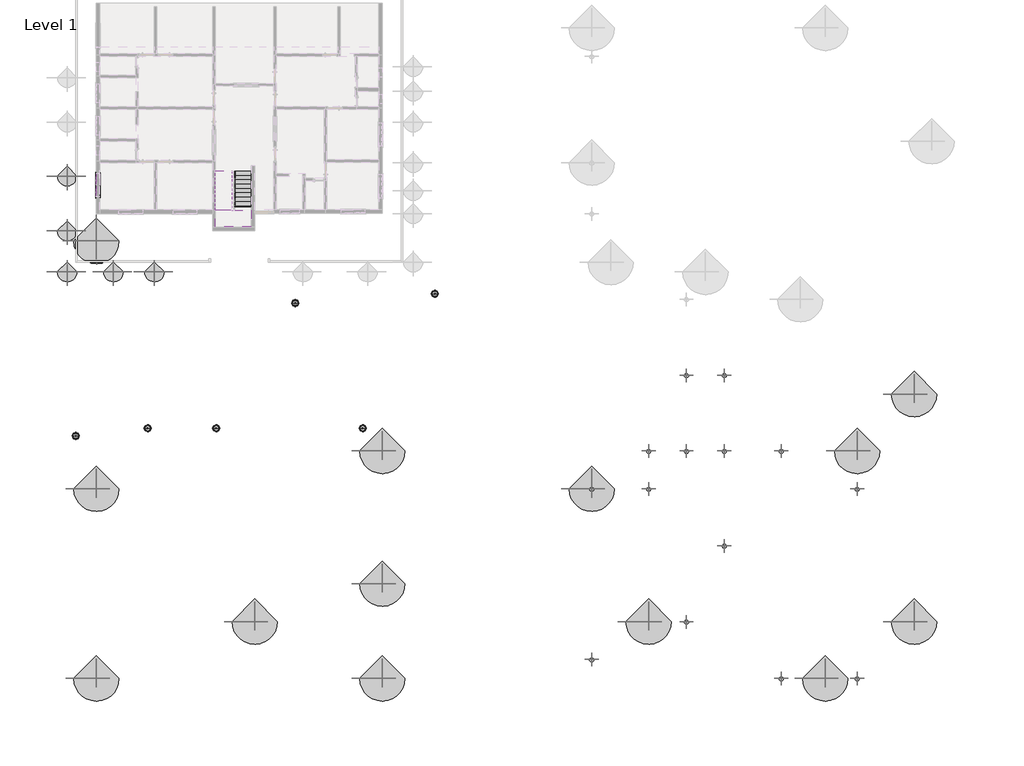
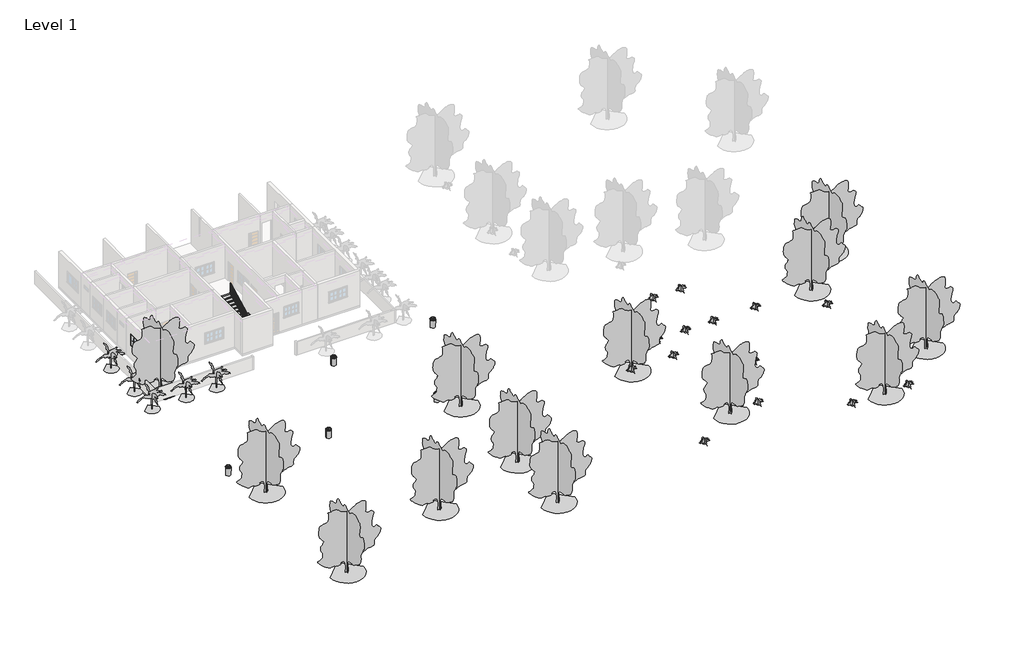
# One storey, part 4 of 5: 32 geographic elements, 10 proxies, 2 stair flights, 1 railing, 1 slab.
"""IFC4 building model written with IfcOpenShell, lengths in millimetres."""

from ifc_helpers import new_model, si_unit, frame, origin, place, context, project, spatial, polyline, outline, extrude, faceted_brep, transform, mapped, element, save
from components import m_muntin_pattern_2x2_m_muntin_pattern_2x2_9352d081, m_muntin_pattern_2x2_m_muntin_pattern_2x2_5c2cbe28, m_recycle_bin_round_m_recycle_bin_round_6e7ed866, m_trim_window_exterior_flat_with_sill_e3533f3c, m_trim_window_interior_flat_picture_frame_7d8195fd, m_rpc_plant_tropical_agave_0_45_meters_eb57889b, m_rpc_tree_tropical_australian_tree_fern_1_8_meters_0203a3dd, rpc_tree_deciduous_american_beech_20_b3c041c8, non_monolithic_landing_4bbdd230, stair_flight_1f098d2d, stair_flight_df8bf18d

model = new_model("IFC4")

# Units and contexts
model_context = context("Model", 3, world=origin())
ifc_project = project(units=[si_unit("LENGTHUNIT", "METRE", prefix="MILLI")], contexts=[model_context])

# Site, building, storey
site = spatial("IfcSite", under=ifc_project)
building = spatial("IfcBuilding", under=site)
storey = spatial("IfcBuildingStorey", under=building, Name="Level 1", Elevation=0.0)

# Proxies
placement = place(None, origin())
m_muntin_pattern_2x2_m_muntin_pattern_2x2_shape = m_muntin_pattern_2x2_m_muntin_pattern_2x2_9352d081(model_context)
element("IfcBuildingElementProxy", 1, Name="M_Muntin Pattern_2x2 : M_Muntin Pattern_2x2", ObjectType="M_Muntin Pattern_2x2 : M_Muntin Pattern_2x2", at=placement, inside=storey, context=model_context, shape_type="MappedRepresentation", body=[
    mapped(m_muntin_pattern_2x2_m_muntin_pattern_2x2_shape, transform((-24995.1597893, 11242.1797903, 1289.0070312), x_axis=(0.0, 1.0, 0.0), y_axis=(-1.0, 0.0, 0.0), z_axis=(0.0, 0.0, 1.0))),
])
m_muntin_pattern_2x2_m_muntin_pattern_2x2_2_shape = m_muntin_pattern_2x2_m_muntin_pattern_2x2_5c2cbe28(model_context)
element("IfcBuildingElementProxy", 2, Name="M_Muntin Pattern_2x2 : M_Muntin Pattern_2x2", ObjectType="M_Muntin Pattern_2x2 : M_Muntin Pattern_2x2", at=placement, inside=storey, context=model_context, shape_type="MappedRepresentation", body=[
    mapped(m_muntin_pattern_2x2_m_muntin_pattern_2x2_2_shape, transform((-24995.1597893, 12001.0047903, 1289.0070313), x_axis=(0.0, -1.0, 0.0), y_axis=(1.0, 0.0, 0.0), z_axis=(0.0, 0.0, 1.0))),
])
m_recycle_bin_round_m_recycle_bin_round_shape = m_recycle_bin_round_m_recycle_bin_round_6e7ed866(model_context)
element("IfcBuildingElementProxy", 3, Name="M_Recycle Bin-Round : M_Recycle Bin-Round", ObjectType="M_Recycle Bin-Round : M_Recycle Bin-Round", at=placement, inside=storey, context=model_context, shape_type="MappedRepresentation", body=[
    mapped(m_recycle_bin_round_m_recycle_bin_round_shape, transform((-21715.3847893, -4012.1077097, 0.0), x_axis=(1.0, 0.0, 0.0), y_axis=(0.0, 1.0, 0.0), z_axis=(0.0, 0.0, 1.0))),
])
element("IfcBuildingElementProxy", 4, Name="M_Recycle Bin-Round : M_Recycle Bin-Round", ObjectType="M_Recycle Bin-Round : M_Recycle Bin-Round", at=placement, inside=storey, context=model_context, shape_type="MappedRepresentation", body=[
    mapped(m_recycle_bin_round_m_recycle_bin_round_shape, transform((-17309.3894725, -4012.1077097, 0.0), x_axis=(1.0, 0.0, 0.0), y_axis=(0.0, 1.0, 0.0), z_axis=(0.0, 0.0, 1.0))),
])
element("IfcBuildingElementProxy", 5, Name="M_Recycle Bin-Round : M_Recycle Bin-Round", ObjectType="M_Recycle Bin-Round : M_Recycle Bin-Round", at=placement, inside=storey, context=model_context, shape_type="MappedRepresentation", body=[
    mapped(m_recycle_bin_round_m_recycle_bin_round_shape, transform((-26325.4847893, -4511.9903076, 0.0), x_axis=(1.0, 0.0, 0.0), y_axis=(0.0, 1.0, 0.0), z_axis=(0.0, 0.0, 1.0))),
])
element("IfcBuildingElementProxy", 6, Name="M_Recycle Bin-Round : M_Recycle Bin-Round", ObjectType="M_Recycle Bin-Round : M_Recycle Bin-Round", at=placement, inside=storey, context=model_context, shape_type="MappedRepresentation", body=[
    mapped(m_recycle_bin_round_m_recycle_bin_round_shape, transform((-7879.6394725, -4012.1077097, 0.0), x_axis=(1.0, 0.0, 0.0), y_axis=(0.0, 1.0, 0.0), z_axis=(0.0, 0.0, 1.0))),
])
element("IfcBuildingElementProxy", 7, Name="M_Recycle Bin-Round : M_Recycle Bin-Round", ObjectType="M_Recycle Bin-Round : M_Recycle Bin-Round", at=placement, inside=storey, context=model_context, shape_type="MappedRepresentation", body=[
    mapped(m_recycle_bin_round_m_recycle_bin_round_shape, transform((-3234.4799408, 4623.2115754, 0.0), x_axis=(1.0, 0.0, 0.0), y_axis=(0.0, 1.0, 0.0), z_axis=(0.0, 0.0, 1.0))),
])
element("IfcBuildingElementProxy", 8, Name="M_Recycle Bin-Round : M_Recycle Bin-Round", ObjectType="M_Recycle Bin-Round : M_Recycle Bin-Round", at=placement, inside=storey, context=model_context, shape_type="MappedRepresentation", body=[
    mapped(m_recycle_bin_round_m_recycle_bin_round_shape, transform((-12215.7847893, 4039.6922903, 0.0), x_axis=(1.0, 0.0, 0.0), y_axis=(0.0, 1.0, 0.0), z_axis=(0.0, 0.0, 1.0))),
])
m_trim_window_exterior_flat_with_sill_shape = m_trim_window_exterior_flat_with_sill_e3533f3c(model_context)
element("IfcBuildingElementProxy", 9, Name="M_Trim-Window-Exterior-Flat : with Sill", ObjectType="M_Trim-Window-Exterior-Flat : with Sill", at=placement, inside=storey, context=model_context, shape_type="MappedRepresentation", body=[
    mapped(m_trim_window_exterior_flat_with_sill_shape, transform((-25004.6847893, 11621.5922903, 2133.5570313), x_axis=(0.0, -1.0, 0.0), y_axis=(0.0, 0.0, 1.0), z_axis=(-1.0, 0.0, 0.0))),
])
m_trim_window_interior_flat_picture_frame_shape = m_trim_window_interior_flat_picture_frame_7d8195fd(model_context)
element("IfcBuildingElementProxy", 10, Name="M_Trim-Window-Interior-Flat : Picture Frame", ObjectType="M_Trim-Window-Interior-Flat : Picture Frame", at=placement, inside=storey, context=model_context, shape_type="MappedRepresentation", body=[
    mapped(m_trim_window_interior_flat_picture_frame_shape, transform((-24776.0847893, 11621.5922903, 2133.5570313), x_axis=(0.0, 1.0, 0.0), y_axis=(0.0, 0.0, 1.0), z_axis=(1.0, 0.0, 0.0))),
])

# Geographic elements
m_rpc_plant_tropical_agave_0_45_meters_shape = m_rpc_plant_tropical_agave_0_45_meters_eb57889b(model_context)
element("IfcGeographicElement", 11, ObjectType="M_RPC Plant - Tropical : Agave - 0.45 Meters", at=placement, inside=storey, context=model_context, shape_type="MappedRepresentation", body=[
    mapped(m_rpc_plant_tropical_agave_0_45_meters_shape, transform((12942.7185396, -595.8077097, 0.0), x_axis=(1.0, 0.0, 0.0), y_axis=(0.0, 1.0, 0.0), z_axis=(0.0, 0.0, 1.0))),
])
element("IfcGeographicElement", 12, ObjectType="M_RPC Plant - Tropical : Agave - 0.45 Meters", at=placement, inside=storey, context=model_context, shape_type="MappedRepresentation", body=[
    mapped(m_rpc_plant_tropical_agave_0_45_meters_shape, transform((10504.3185396, -5472.6077097, 0.0), x_axis=(1.0, 0.0, 0.0), y_axis=(0.0, 1.0, 0.0), z_axis=(0.0, 0.0, 1.0))),
])
element("IfcGeographicElement", 13, ObjectType="M_RPC Plant - Tropical : Agave - 0.45 Meters", at=placement, inside=storey, context=model_context, shape_type="MappedRepresentation", body=[
    mapped(m_rpc_plant_tropical_agave_0_45_meters_shape, transform((6846.7185396, -7911.0077097, 0.0), x_axis=(1.0, 0.0, 0.0), y_axis=(0.0, 1.0, 0.0), z_axis=(0.0, 0.0, 1.0))),
])
element("IfcGeographicElement", 14, ObjectType="M_RPC Plant - Tropical : Agave - 0.45 Meters", at=placement, inside=storey, context=model_context, shape_type="MappedRepresentation", body=[
    mapped(m_rpc_plant_tropical_agave_0_45_meters_shape, transform((15381.1185396, -5472.6077097, 0.0), x_axis=(1.0, 0.0, 0.0), y_axis=(0.0, 1.0, 0.0), z_axis=(0.0, 0.0, 1.0))),
])
element("IfcGeographicElement", 15, ObjectType="M_RPC Plant - Tropical : Agave - 0.45 Meters", at=placement, inside=storey, context=model_context, shape_type="MappedRepresentation", body=[
    mapped(m_rpc_plant_tropical_agave_0_45_meters_shape, transform((19038.7185396, -20103.0077097, 0.0), x_axis=(1.0, 0.0, 0.0), y_axis=(0.0, 1.0, 0.0), z_axis=(0.0, 0.0, 1.0))),
])
element("IfcGeographicElement", 16, ObjectType="M_RPC Plant - Tropical : Agave - 0.45 Meters", at=placement, inside=storey, context=model_context, shape_type="MappedRepresentation", body=[
    mapped(m_rpc_plant_tropical_agave_0_45_meters_shape, transform((15381.1185396, -11568.6077097, 0.0), x_axis=(1.0, 0.0, 0.0), y_axis=(0.0, 1.0, 0.0), z_axis=(0.0, 0.0, 1.0))),
])
element("IfcGeographicElement", 17, ObjectType="M_RPC Plant - Tropical : Agave - 0.45 Meters", at=placement, inside=storey, context=model_context, shape_type="MappedRepresentation", body=[
    mapped(m_rpc_plant_tropical_agave_0_45_meters_shape, transform((19038.7185396, -5472.6077097, 0.0), x_axis=(1.0, 0.0, 0.0), y_axis=(0.0, 1.0, 0.0), z_axis=(0.0, 0.0, 1.0))),
])
element("IfcGeographicElement", 18, ObjectType="M_RPC Plant - Tropical : Agave - 0.45 Meters", at=placement, inside=storey, context=model_context, shape_type="MappedRepresentation", body=[
    mapped(m_rpc_plant_tropical_agave_0_45_meters_shape, transform((23915.5185396, -7911.0077097, 0.0), x_axis=(1.0, 0.0, 0.0), y_axis=(0.0, 1.0, 0.0), z_axis=(0.0, 0.0, 1.0))),
])
element("IfcGeographicElement", 19, ObjectType="M_RPC Plant - Tropical : Agave - 0.45 Meters", at=placement, inside=storey, context=model_context, shape_type="MappedRepresentation", body=[
    mapped(m_rpc_plant_tropical_agave_0_45_meters_shape, transform((23915.5185396, -20103.0077097, 0.0), x_axis=(1.0, 0.0, 0.0), y_axis=(0.0, 1.0, 0.0), z_axis=(0.0, 0.0, 1.0))),
])
element("IfcGeographicElement", 20, ObjectType="M_RPC Plant - Tropical : Agave - 0.45 Meters", at=placement, inside=storey, context=model_context, shape_type="MappedRepresentation", body=[
    mapped(m_rpc_plant_tropical_agave_0_45_meters_shape, transform((12942.7185396, -16445.4077097, 0.0), x_axis=(1.0, 0.0, 0.0), y_axis=(0.0, 1.0, 0.0), z_axis=(0.0, 0.0, 1.0))),
])
element("IfcGeographicElement", 21, ObjectType="M_RPC Plant - Tropical : Agave - 0.45 Meters", at=placement, inside=storey, context=model_context, shape_type="MappedRepresentation", body=[
    mapped(m_rpc_plant_tropical_agave_0_45_meters_shape, transform((6846.7185396, -18883.8077097, 0.0), x_axis=(1.0, 0.0, 0.0), y_axis=(0.0, 1.0, 0.0), z_axis=(0.0, 0.0, 1.0))),
])
element("IfcGeographicElement", 22, ObjectType="M_RPC Plant - Tropical : Agave - 0.45 Meters", at=placement, inside=storey, context=model_context, shape_type="MappedRepresentation", body=[
    mapped(m_rpc_plant_tropical_agave_0_45_meters_shape, transform((10504.3185396, -7911.0077097, 0.0), x_axis=(1.0, 0.0, 0.0), y_axis=(0.0, 1.0, 0.0), z_axis=(0.0, 0.0, 1.0))),
])
element("IfcGeographicElement", 23, ObjectType="M_RPC Plant - Tropical : Agave - 0.45 Meters", at=placement, inside=storey, context=model_context, shape_type="MappedRepresentation", body=[
    mapped(m_rpc_plant_tropical_agave_0_45_meters_shape, transform((12942.7185396, -5472.6077097, 0.0), x_axis=(1.0, 0.0, 0.0), y_axis=(0.0, 1.0, 0.0), z_axis=(0.0, 0.0, 1.0))),
])
element("IfcGeographicElement", 24, ObjectType="M_RPC Plant - Tropical : Agave - 0.45 Meters", at=placement, inside=storey, context=model_context, shape_type="MappedRepresentation", body=[
    mapped(m_rpc_plant_tropical_agave_0_45_meters_shape, transform((15381.1185396, -595.8077097, 0.0), x_axis=(1.0, 0.0, 0.0), y_axis=(0.0, 1.0, 0.0), z_axis=(0.0, 0.0, 1.0))),
])
m_rpc_tree_tropical_australian_tree_fern_1_8_meters_shape = m_rpc_tree_tropical_australian_tree_fern_1_8_meters_0203a3dd(model_context)
element("IfcGeographicElement", 25, ObjectType="M_RPC Tree - Tropical : Australian Tree Fern - 1.8 Meters", at=placement, inside=storey, context=model_context, shape_type="MappedRepresentation", body=[
    mapped(m_rpc_tree_tropical_australian_tree_fern_1_8_meters_shape, transform((-26884.4814604, 12205.7922903, -152.4), x_axis=(1.0, 0.0, 0.0), y_axis=(0.0, 1.0, 0.0), z_axis=(0.0, 0.0, 1.0))),
])
element("IfcGeographicElement", 26, ObjectType="M_RPC Tree - Tropical : Australian Tree Fern - 1.8 Meters", at=placement, inside=storey, context=model_context, shape_type="MappedRepresentation", body=[
    mapped(m_rpc_tree_tropical_australian_tree_fern_1_8_meters_shape, transform((-26884.4814604, 8675.1922903, -152.4), x_axis=(1.0, 0.0, 0.0), y_axis=(0.0, 1.0, 0.0), z_axis=(0.0, 0.0, 1.0))),
])
element("IfcGeographicElement", 27, ObjectType="M_RPC Tree - Tropical : Australian Tree Fern - 1.8 Meters", at=placement, inside=storey, context=model_context, shape_type="MappedRepresentation", body=[
    mapped(m_rpc_tree_tropical_australian_tree_fern_1_8_meters_shape, transform((-26884.4814604, 6035.3596924, -152.4), x_axis=(1.0, 0.0, 0.0), y_axis=(0.0, 1.0, 0.0), z_axis=(0.0, 0.0, 1.0))),
])
element("IfcGeographicElement", 28, ObjectType="M_RPC Tree - Tropical : Australian Tree Fern - 1.8 Meters", at=placement, inside=storey, context=model_context, shape_type="MappedRepresentation", body=[
    mapped(m_rpc_tree_tropical_australian_tree_fern_1_8_meters_shape, transform((-21271.0814604, 6035.3596924, -152.4), x_axis=(1.0, 0.0, 0.0), y_axis=(0.0, 1.0, 0.0), z_axis=(0.0, 0.0, 1.0))),
])
element("IfcGeographicElement", 29, ObjectType="M_RPC Tree - Tropical : Australian Tree Fern - 1.8 Meters", at=placement, inside=storey, context=model_context, shape_type="MappedRepresentation", body=[
    mapped(m_rpc_tree_tropical_australian_tree_fern_1_8_meters_shape, transform((-23910.4111436, 6035.3596924, -152.4), x_axis=(1.0, 0.0, 0.0), y_axis=(0.0, 1.0, 0.0), z_axis=(0.0, 0.0, 1.0))),
])
rpc_tree_deciduous_american_beech_20_shape = rpc_tree_deciduous_american_beech_20_b3c041c8(model_context)
element("IfcGeographicElement", 30, ObjectType="RPC Tree - Deciduous : American Beech - 20'", at=placement, inside=storey, context=model_context, shape_type="MappedRepresentation", body=[
    mapped(rpc_tree_deciduous_american_beech_20_shape, transform((27573.3152107, -1815.0077097, 0.0), x_axis=(1.0, 0.0, 0.0), y_axis=(0.0, 1.0, 0.0), z_axis=(0.0, 0.0, 1.0))),
])
element("IfcGeographicElement", 31, ObjectType="RPC Tree - Deciduous : American Beech - 20'", at=placement, inside=storey, context=model_context, shape_type="MappedRepresentation", body=[
    mapped(rpc_tree_deciduous_american_beech_20_shape, transform((21866.0890435, -20103.0077097, 0.0), x_axis=(1.0, 0.0, 0.0), y_axis=(0.0, 1.0, 0.0), z_axis=(0.0, 0.0, 1.0))),
])
element("IfcGeographicElement", 32, ObjectType="RPC Tree - Deciduous : American Beech - 20'", at=placement, inside=storey, context=model_context, shape_type="MappedRepresentation", body=[
    mapped(rpc_tree_deciduous_american_beech_20_shape, transform((27573.3152107, -16445.4077097, 0.0), x_axis=(1.0, 0.0, 0.0), y_axis=(0.0, 1.0, 0.0), z_axis=(0.0, 0.0, 1.0))),
])
element("IfcGeographicElement", 33, ObjectType="RPC Tree - Deciduous : American Beech - 20'", at=placement, inside=storey, context=model_context, shape_type="MappedRepresentation", body=[
    mapped(rpc_tree_deciduous_american_beech_20_shape, transform((23915.7152107, -5472.6077097, 0.0), x_axis=(1.0, 0.0, 0.0), y_axis=(0.0, 1.0, 0.0), z_axis=(0.0, 0.0, 1.0))),
])
element("IfcGeographicElement", 34, ObjectType="RPC Tree - Deciduous : American Beech - 20'", at=placement, inside=storey, context=model_context, shape_type="MappedRepresentation", body=[
    mapped(rpc_tree_deciduous_american_beech_20_shape, transform((6846.9152107, -7911.0077097, 0.0), x_axis=(1.0, 0.0, 0.0), y_axis=(0.0, 1.0, 0.0), z_axis=(0.0, 0.0, 1.0))),
])
element("IfcGeographicElement", 35, ObjectType="RPC Tree - Deciduous : American Beech - 20'", at=placement, inside=storey, context=model_context, shape_type="MappedRepresentation", body=[
    mapped(rpc_tree_deciduous_american_beech_20_shape, transform((10504.5152107, -16445.4077097, 0.0), x_axis=(1.0, 0.0, 0.0), y_axis=(0.0, 1.0, 0.0), z_axis=(0.0, 0.0, 1.0))),
])
element("IfcGeographicElement", 36, ObjectType="RPC Tree - Deciduous : American Beech - 20'", at=placement, inside=storey, context=model_context, shape_type="MappedRepresentation", body=[
    mapped(rpc_tree_deciduous_american_beech_20_shape, transform((-25004.6847893, -7911.0077097, 0.0), x_axis=(1.0, 0.0, 0.0), y_axis=(0.0, 1.0, 0.0), z_axis=(0.0, 0.0, 1.0))),
])
element("IfcGeographicElement", 37, ObjectType="RPC Tree - Deciduous : American Beech - 20'", at=placement, inside=storey, context=model_context, shape_type="MappedRepresentation", body=[
    mapped(rpc_tree_deciduous_american_beech_20_shape, transform((-6615.0847893, -5472.6077097, 0.0), x_axis=(1.0, 0.0, 0.0), y_axis=(0.0, 1.0, 0.0), z_axis=(0.0, 0.0, 1.0))),
])
element("IfcGeographicElement", 38, ObjectType="RPC Tree - Deciduous : American Beech - 20'", at=placement, inside=storey, context=model_context, shape_type="MappedRepresentation", body=[
    mapped(rpc_tree_deciduous_american_beech_20_shape, transform((-6615.0847893, -14007.0077097, 0.0), x_axis=(1.0, 0.0, 0.0), y_axis=(0.0, 1.0, 0.0), z_axis=(0.0, 0.0, 1.0))),
])
element("IfcGeographicElement", 39, ObjectType="RPC Tree - Deciduous : American Beech - 20'", at=placement, inside=storey, context=model_context, shape_type="MappedRepresentation", body=[
    mapped(rpc_tree_deciduous_american_beech_20_shape, transform((-6615.0847893, -20103.0077097, 0.0), x_axis=(1.0, 0.0, 0.0), y_axis=(0.0, 1.0, 0.0), z_axis=(0.0, 0.0, 1.0))),
])
element("IfcGeographicElement", 40, ObjectType="RPC Tree - Deciduous : American Beech - 20'", at=placement, inside=storey, context=model_context, shape_type="MappedRepresentation", body=[
    mapped(rpc_tree_deciduous_american_beech_20_shape, transform((-25004.6847893, -20103.0077097, 0.0), x_axis=(1.0, 0.0, 0.0), y_axis=(0.0, 1.0, 0.0), z_axis=(0.0, 0.0, 1.0))),
])
element("IfcGeographicElement", 41, ObjectType="RPC Tree - Deciduous : American Beech - 20'", at=placement, inside=storey, context=model_context, shape_type="MappedRepresentation", body=[
    mapped(rpc_tree_deciduous_american_beech_20_shape, transform((-14819.2847893, -16445.4077097, 0.0), x_axis=(1.0, 0.0, 0.0), y_axis=(0.0, 1.0, 0.0), z_axis=(0.0, 0.0, 1.0))),
])
element("IfcGeographicElement", 42, ObjectType="RPC Tree - Deciduous : American Beech - 20'", at=placement, inside=storey, context=model_context, shape_type="MappedRepresentation", body=[
    mapped(rpc_tree_deciduous_american_beech_20_shape, transform((-25004.6847893, 8027.4922903, -152.4), x_axis=(1.0, 0.0, 0.0), y_axis=(0.0, 1.0, 0.0), z_axis=(0.0, 0.0, 1.0))),
])

# Railing
element("IfcRailing", 43, ObjectType="Handrail - Rectangular", at=placement, inside=storey, context=model_context, shape_type="SolidModel", body=[
    faceted_brep([(-16063.8847893, 12510.5922903, 1059.8727273), (-16063.8847893, 12510.5922903, 1002.5995168), (-16114.6847893, 12510.5922903, 1002.5995168), (-16114.6847893, 12510.5922903, 1059.8727273), (-16063.8847893, 10072.1922903, 2329.4528926), (-16063.8847893, 10021.3922903, 2298.6292688), (-16114.6847893, 10021.3922903, 2298.6292688), (-16114.6847893, 10072.1922903, 2329.4528926), (-16063.8847893, 10072.1922903, 2369.1272727), (-16063.8847893, 10021.3922903, 2318.3272727), (-16114.6847893, 10021.3922903, 2318.3272727), (-16114.6847893, 10072.1922903, 2369.1272727), (-16063.8847893, 9945.1922903, 2369.1272727), (-16063.8847893, 9945.1922903, 2318.3272727), (-16114.6847893, 9995.9922903, 2318.3272727), (-16114.6847893, 9995.9922903, 2369.1272727), (-16190.8847893, 9945.1922903, 2369.1272727), (-16190.8847893, 9945.1922903, 2318.3272727), (-16190.8847893, 9995.9922903, 2318.3272727), (-16190.8847893, 9995.9922903, 2369.1272727), (-16216.2847893, 9945.1922903, 2369.1272727), (-16267.0847893, 9945.1922903, 2318.3272727), (-16267.0847893, 9995.9922903, 2318.3272727), (-16216.2847893, 9995.9922903, 2369.1272727), (-16216.2847893, 9945.1922903, 2554.2743802), (-16267.0847893, 9945.1922903, 2503.4743802), (-16267.0847893, 9995.9922903, 2503.4743802), (-16216.2847893, 9995.9922903, 2554.2743802), (-16343.2847893, 9945.1922903, 2554.2743802), (-16343.2847893, 9945.1922903, 2503.4743802), (-16292.4847893, 9995.9922903, 2503.4743802), (-16292.4847893, 9995.9922903, 2554.2743802), (-16343.2847893, 10072.1922903, 2554.2743802), (-16343.2847893, 10084.6249644, 2503.4743802), (-16292.4847893, 10084.6249644, 2503.4743802), (-16292.4847893, 10072.1922903, 2554.2743802), (-16343.2847893, 12510.5922903, 3823.8545455), (-16292.4847893, 12510.5922903, 3823.8545455), (-16292.4847893, 12510.5922903, 3766.581335), (-16343.2847893, 12510.5922903, 3766.581335)], [[[0, 1, 2, 3]], [[1, 0, 4, 5]], [[2, 1, 5, 6]], [[3, 2, 6, 7]], [[0, 3, 7, 4]], [[5, 4, 8, 9]], [[6, 5, 9, 10]], [[7, 6, 10, 11]], [[4, 7, 11, 8]], [[9, 8, 12, 13]], [[10, 9, 13, 14]], [[11, 10, 14, 15]], [[8, 11, 15, 12]], [[13, 12, 16, 17]], [[14, 13, 17, 18]], [[15, 14, 18, 19]], [[12, 15, 19, 16]], [[17, 16, 20, 21]], [[18, 17, 21, 22]], [[19, 18, 22, 23]], [[16, 19, 23, 20]], [[21, 20, 24, 25]], [[22, 21, 25, 26]], [[23, 22, 26, 27]], [[20, 23, 27, 24]], [[25, 24, 28, 29]], [[26, 25, 29, 30]], [[27, 26, 30, 31]], [[24, 27, 31, 28]], [[29, 28, 32, 33]], [[30, 29, 33, 34]], [[31, 30, 34, 35]], [[28, 31, 35, 32]], [[36, 37, 38, 39]], [[33, 32, 36, 39]], [[34, 33, 39, 38]], [[35, 34, 38, 37]], [[32, 35, 37, 36]]]),
    extrude(outline(polyline([(12399.4672903, 3708.7228639), (12418.5172903, 3718.6414589), (12418.5172903, 2763.9818182), (12399.4672903, 2763.9818182), (12399.4672903, 3708.7228639)])), frame((-16327.4097893, 0.0, 0.0), z_axis=(1.0, 0.0, 0.0), x_axis=(0.0, 1.0, 0.0)), (0.0, 0.0, 1.0), 19.05),
    extrude(outline(polyline([(12297.8672903, 3655.8236903), (12316.9172903, 3665.7422854), (12316.9172903, 2763.9818182), (12297.8672903, 2763.9818182), (12297.8672903, 3655.8236903)])), frame((-16327.4097893, 0.0, 0.0), z_axis=(1.0, 0.0, 0.0), x_axis=(0.0, 1.0, 0.0)), (0.0, 0.0, 1.0), 19.05),
    extrude(outline(polyline([(12196.2672903, 3602.9245168), (12215.3172903, 3612.8431118), (12215.3172903, 2618.5090909), (12196.2672903, 2618.5090909), (12196.2672903, 3602.9245168)])), frame((-16327.4097893, 0.0, 0.0), z_axis=(1.0, 0.0, 0.0), x_axis=(0.0, 1.0, 0.0)), (0.0, 0.0, 1.0), 19.05),
    extrude(outline(polyline([(12094.6672903, 3550.0253432), (12113.7172903, 3559.9439383), (12113.7172903, 2618.5090909), (12094.6672903, 2618.5090909), (12094.6672903, 3550.0253432)])), frame((-16327.4097893, 0.0, 0.0), z_axis=(1.0, 0.0, 0.0), x_axis=(0.0, 1.0, 0.0)), (0.0, 0.0, 1.0), 19.05),
    extrude(outline(polyline([(11993.0672903, 3497.1261697), (12012.1172903, 3507.0447647), (12012.1172903, 2618.5090909), (11993.0672903, 2618.5090909), (11993.0672903, 3497.1261697)])), frame((-16327.4097893, 0.0, 0.0), z_axis=(1.0, 0.0, 0.0), x_axis=(0.0, 1.0, 0.0)), (0.0, 0.0, 1.0), 19.05),
    extrude(outline(polyline([(11891.4672903, 3444.2269961), (11910.5172903, 3454.1455912), (11910.5172903, 2473.0363636), (11891.4672903, 2473.0363636), (11891.4672903, 3444.2269961)])), frame((-16327.4097893, 0.0, 0.0), z_axis=(1.0, 0.0, 0.0), x_axis=(0.0, 1.0, 0.0)), (0.0, 0.0, 1.0), 19.05),
    extrude(outline(polyline([(11789.8672903, 3391.3278226), (11808.9172903, 3401.2464176), (11808.9172903, 2473.0363636), (11789.8672903, 2473.0363636), (11789.8672903, 3391.3278226)])), frame((-16327.4097893, 0.0, 0.0), z_axis=(1.0, 0.0, 0.0), x_axis=(0.0, 1.0, 0.0)), (0.0, 0.0, 1.0), 19.05),
    extrude(outline(polyline([(11688.2672903, 3338.428649), (11707.3172903, 3348.347244), (11707.3172903, 2473.0363636), (11688.2672903, 2473.0363636), (11688.2672903, 3338.428649)])), frame((-16327.4097893, 0.0, 0.0), z_axis=(1.0, 0.0, 0.0), x_axis=(0.0, 1.0, 0.0)), (0.0, 0.0, 1.0), 19.05),
    extrude(outline(polyline([(11586.6672903, 3285.5294755), (11605.7172903, 3295.4480705), (11605.7172903, 2327.5636364), (11586.6672903, 2327.5636364), (11586.6672903, 3285.5294755)])), frame((-16327.4097893, 0.0, 0.0), z_axis=(1.0, 0.0, 0.0), x_axis=(0.0, 1.0, 0.0)), (0.0, 0.0, 1.0), 19.05),
    extrude(outline(polyline([(11485.0672903, 3232.6303019), (11504.1172903, 3242.5488969), (11504.1172903, 2327.5636364), (11485.0672903, 2327.5636364), (11485.0672903, 3232.6303019)])), frame((-16327.4097893, 0.0, 0.0), z_axis=(1.0, 0.0, 0.0), x_axis=(0.0, 1.0, 0.0)), (0.0, 0.0, 1.0), 19.05),
    extrude(outline(polyline([(11383.4672903, 3179.7311283), (11402.5172903, 3189.6497234), (11402.5172903, 2327.5636364), (11383.4672903, 2327.5636364), (11383.4672903, 3179.7311283)])), frame((-16327.4097893, 0.0, 0.0), z_axis=(1.0, 0.0, 0.0), x_axis=(0.0, 1.0, 0.0)), (0.0, 0.0, 1.0), 19.05),
    extrude(outline(polyline([(11281.8672903, 3126.8319548), (11300.9172903, 3136.7505498), (11300.9172903, 2182.0909091), (11281.8672903, 2182.0909091), (11281.8672903, 3126.8319548)])), frame((-16327.4097893, 0.0, 0.0), z_axis=(1.0, 0.0, 0.0), x_axis=(0.0, 1.0, 0.0)), (0.0, 0.0, 1.0), 19.05),
    extrude(outline(polyline([(11180.2672903, 3073.9327812), (11199.3172903, 3083.8513763), (11199.3172903, 2182.0909091), (11180.2672903, 2182.0909091), (11180.2672903, 3073.9327812)])), frame((-16327.4097893, 0.0, 0.0), z_axis=(1.0, 0.0, 0.0), x_axis=(0.0, 1.0, 0.0)), (0.0, 0.0, 1.0), 19.05),
    extrude(outline(polyline([(11078.6672903, 3021.0336077), (11097.7172903, 3030.9522027), (11097.7172903, 2036.6181818), (11078.6672903, 2036.6181818), (11078.6672903, 3021.0336077)])), frame((-16327.4097893, 0.0, 0.0), z_axis=(1.0, 0.0, 0.0), x_axis=(0.0, 1.0, 0.0)), (0.0, 0.0, 1.0), 19.05),
    extrude(outline(polyline([(10977.0672903, 2968.1344341), (10996.1172903, 2978.0530292), (10996.1172903, 2036.6181818), (10977.0672903, 2036.6181818), (10977.0672903, 2968.1344341)])), frame((-16327.4097893, 0.0, 0.0), z_axis=(1.0, 0.0, 0.0), x_axis=(0.0, 1.0, 0.0)), (0.0, 0.0, 1.0), 19.05),
    extrude(outline(polyline([(10875.4672903, 2915.2352606), (10894.5172903, 2925.1538556), (10894.5172903, 2036.6181818), (10875.4672903, 2036.6181818), (10875.4672903, 2915.2352606)])), frame((-16327.4097893, 0.0, 0.0), z_axis=(1.0, 0.0, 0.0), x_axis=(0.0, 1.0, 0.0)), (0.0, 0.0, 1.0), 19.05),
    extrude(outline(polyline([(10773.8672903, 2862.336087), (10792.9172903, 2872.2546821), (10792.9172903, 1891.1454545), (10773.8672903, 1891.1454545), (10773.8672903, 2862.336087)])), frame((-16327.4097893, 0.0, 0.0), z_axis=(1.0, 0.0, 0.0), x_axis=(0.0, 1.0, 0.0)), (0.0, 0.0, 1.0), 19.05),
    extrude(outline(polyline([(10672.2672903, 2809.4369135), (10691.3172903, 2819.3555085), (10691.3172903, 1891.1454545), (10672.2672903, 1891.1454545), (10672.2672903, 2809.4369135)])), frame((-16327.4097893, 0.0, 0.0), z_axis=(1.0, 0.0, 0.0), x_axis=(0.0, 1.0, 0.0)), (0.0, 0.0, 1.0), 19.05),
    extrude(outline(polyline([(10570.6672903, 2756.5377399), (10589.7172903, 2766.456335), (10589.7172903, 1891.1454545), (10570.6672903, 1891.1454545), (10570.6672903, 2756.5377399)])), frame((-16327.4097893, 0.0, 0.0), z_axis=(1.0, 0.0, 0.0), x_axis=(0.0, 1.0, 0.0)), (0.0, 0.0, 1.0), 19.05),
    extrude(outline(polyline([(10469.0672903, 2703.6385664), (10488.1172903, 2713.5571614), (10488.1172903, 1745.6727273), (10469.0672903, 1745.6727273), (10469.0672903, 2703.6385664)])), frame((-16327.4097893, 0.0, 0.0), z_axis=(1.0, 0.0, 0.0), x_axis=(0.0, 1.0, 0.0)), (0.0, 0.0, 1.0), 19.05),
    extrude(outline(polyline([(10367.4672903, 2650.7393928), (10386.5172903, 2660.6579878), (10386.5172903, 1745.6727273), (10367.4672903, 1745.6727273), (10367.4672903, 2650.7393928)])), frame((-16327.4097893, 0.0, 0.0), z_axis=(1.0, 0.0, 0.0), x_axis=(0.0, 1.0, 0.0)), (0.0, 0.0, 1.0), 19.05),
    extrude(outline(polyline([(10265.8672903, 2597.8402193), (10284.9172903, 2607.7588143), (10284.9172903, 1745.6727273), (10265.8672903, 1745.6727273), (10265.8672903, 2597.8402193)])), frame((-16327.4097893, 0.0, 0.0), z_axis=(1.0, 0.0, 0.0), x_axis=(0.0, 1.0, 0.0)), (0.0, 0.0, 1.0), 19.05),
    extrude(outline(polyline([(10164.2672903, 2544.9410457), (10183.3172903, 2554.8596407), (10183.3172903, 1600.2), (10164.2672903, 1600.2), (10164.2672903, 2544.9410457)])), frame((-16327.4097893, 0.0, 0.0), z_axis=(1.0, 0.0, 0.0), x_axis=(0.0, 1.0, 0.0)), (0.0, 0.0, 1.0), 19.05),
    extrude(outline(polyline([(10062.6672903, 2492.0418721), (10081.7172903, 2501.9604672), (10081.7172903, 1600.2), (10062.6672903, 1600.2), (10062.6672903, 2492.0418721)])), frame((-16327.4097893, 0.0, 0.0), z_axis=(1.0, 0.0, 0.0), x_axis=(0.0, 1.0, 0.0)), (0.0, 0.0, 1.0), 19.05),
    extrude(outline(polyline([(-16282.9597893, 9980.1172903), (-16282.9597893, 9961.0672903), (-16302.0097893, 9961.0672903), (-16302.0097893, 9980.1172903), (-16282.9597893, 9980.1172903)])), frame((0.0, 0.0, 1454.7272727), z_axis=(0.0, 0.0, 1.0), x_axis=(1.0, 0.0, 0.0)), (0.0, 0.0, 1.0), 1048.7471074),
    extrude(outline(polyline([(-16181.3597893, 9980.1172903), (-16181.3597893, 9961.0672903), (-16200.4097893, 9961.0672903), (-16200.4097893, 9980.1172903), (-16181.3597893, 9980.1172903)])), frame((0.0, 0.0, 1454.7272727), z_axis=(0.0, 0.0, 1.0), x_axis=(1.0, 0.0, 0.0)), (0.0, 0.0, 1.0), 863.6),
    extrude(outline(polyline([(10062.6672903, 2277.1389796), (10081.7172903, 2267.2203845), (10081.7172903, 1309.2545455), (10062.6672903, 1309.2545455), (10062.6672903, 2277.1389796)])), frame((-16098.8097893, 0.0, 0.0), z_axis=(1.0, 0.0, 0.0), x_axis=(0.0, 1.0, 0.0)), (0.0, 0.0, 1.0), 19.05),
    extrude(outline(polyline([(10164.2672903, 2224.239806), (10183.3172903, 2214.321211), (10183.3172903, 1309.2545455), (10164.2672903, 1309.2545455), (10164.2672903, 2224.239806)])), frame((-16098.8097893, 0.0, 0.0), z_axis=(1.0, 0.0, 0.0), x_axis=(0.0, 1.0, 0.0)), (0.0, 0.0, 1.0), 19.05),
    extrude(outline(polyline([(10265.8672903, 2171.3406325), (10284.9172903, 2161.4220374), (10284.9172903, 1309.2545455), (10265.8672903, 1309.2545455), (10265.8672903, 2171.3406325)])), frame((-16098.8097893, 0.0, 0.0), z_axis=(1.0, 0.0, 0.0), x_axis=(0.0, 1.0, 0.0)), (0.0, 0.0, 1.0), 19.05),
    extrude(outline(polyline([(10367.4672903, 2118.4414589), (10386.5172903, 2108.5228639), (10386.5172903, 1163.7818182), (10367.4672903, 1163.7818182), (10367.4672903, 2118.4414589)])), frame((-16098.8097893, 0.0, 0.0), z_axis=(1.0, 0.0, 0.0), x_axis=(0.0, 1.0, 0.0)), (0.0, 0.0, 1.0), 19.05),
    extrude(outline(polyline([(10469.0672903, 2065.5422854), (10488.1172903, 2055.6236903), (10488.1172903, 1163.7818182), (10469.0672903, 1163.7818182), (10469.0672903, 2065.5422854)])), frame((-16098.8097893, 0.0, 0.0), z_axis=(1.0, 0.0, 0.0), x_axis=(0.0, 1.0, 0.0)), (0.0, 0.0, 1.0), 19.05),
    extrude(outline(polyline([(10570.6672903, 2012.6431118), (10589.7172903, 2002.7245168), (10589.7172903, 1018.3090909), (10570.6672903, 1018.3090909), (10570.6672903, 2012.6431118)])), frame((-16098.8097893, 0.0, 0.0), z_axis=(1.0, 0.0, 0.0), x_axis=(0.0, 1.0, 0.0)), (0.0, 0.0, 1.0), 19.05),
    extrude(outline(polyline([(10672.2672903, 1959.7439383), (10691.3172903, 1949.8253432), (10691.3172903, 1018.3090909), (10672.2672903, 1018.3090909), (10672.2672903, 1959.7439383)])), frame((-16098.8097893, 0.0, 0.0), z_axis=(1.0, 0.0, 0.0), x_axis=(0.0, 1.0, 0.0)), (0.0, 0.0, 1.0), 19.05),
    extrude(outline(polyline([(10773.8672903, 1906.8447647), (10792.9172903, 1896.9261697), (10792.9172903, 1018.3090909), (10773.8672903, 1018.3090909), (10773.8672903, 1906.8447647)])), frame((-16098.8097893, 0.0, 0.0), z_axis=(1.0, 0.0, 0.0), x_axis=(0.0, 1.0, 0.0)), (0.0, 0.0, 1.0), 19.05),
    extrude(outline(polyline([(10875.4672903, 1853.9455912), (10894.5172903, 1844.0269961), (10894.5172903, 872.8363636), (10875.4672903, 872.8363636), (10875.4672903, 1853.9455912)])), frame((-16098.8097893, 0.0, 0.0), z_axis=(1.0, 0.0, 0.0), x_axis=(0.0, 1.0, 0.0)), (0.0, 0.0, 1.0), 19.05),
    extrude(outline(polyline([(10977.0672903, 1801.0464176), (10996.1172903, 1791.1278226), (10996.1172903, 872.8363636), (10977.0672903, 872.8363636), (10977.0672903, 1801.0464176)])), frame((-16098.8097893, 0.0, 0.0), z_axis=(1.0, 0.0, 0.0), x_axis=(0.0, 1.0, 0.0)), (0.0, 0.0, 1.0), 19.05),
    extrude(outline(polyline([(11078.6672903, 1748.147244), (11097.7172903, 1738.228649), (11097.7172903, 872.8363636), (11078.6672903, 872.8363636), (11078.6672903, 1748.147244)])), frame((-16098.8097893, 0.0, 0.0), z_axis=(1.0, 0.0, 0.0), x_axis=(0.0, 1.0, 0.0)), (0.0, 0.0, 1.0), 19.05),
    extrude(outline(polyline([(11180.2672903, 1695.2480705), (11199.3172903, 1685.3294755), (11199.3172903, 727.3636364), (11180.2672903, 727.3636364), (11180.2672903, 1695.2480705)])), frame((-16098.8097893, 0.0, 0.0), z_axis=(1.0, 0.0, 0.0), x_axis=(0.0, 1.0, 0.0)), (0.0, 0.0, 1.0), 19.05),
    extrude(outline(polyline([(11281.8672903, 1642.3488969), (11300.9172903, 1632.4303019), (11300.9172903, 727.3636364), (11281.8672903, 727.3636364), (11281.8672903, 1642.3488969)])), frame((-16098.8097893, 0.0, 0.0), z_axis=(1.0, 0.0, 0.0), x_axis=(0.0, 1.0, 0.0)), (0.0, 0.0, 1.0), 19.05),
    extrude(outline(polyline([(11383.4672903, 1589.4497234), (11402.5172903, 1579.5311283), (11402.5172903, 727.3636364), (11383.4672903, 727.3636364), (11383.4672903, 1589.4497234)])), frame((-16098.8097893, 0.0, 0.0), z_axis=(1.0, 0.0, 0.0), x_axis=(0.0, 1.0, 0.0)), (0.0, 0.0, 1.0), 19.05),
    extrude(outline(polyline([(11485.0672903, 1536.5505498), (11504.1172903, 1526.6319548), (11504.1172903, 581.8909091), (11485.0672903, 581.8909091), (11485.0672903, 1536.5505498)])), frame((-16098.8097893, 0.0, 0.0), z_axis=(1.0, 0.0, 0.0), x_axis=(0.0, 1.0, 0.0)), (0.0, 0.0, 1.0), 19.05),
    extrude(outline(polyline([(11586.6672903, 1483.6513763), (11605.7172903, 1473.7327812), (11605.7172903, 581.8909091), (11586.6672903, 581.8909091), (11586.6672903, 1483.6513763)])), frame((-16098.8097893, 0.0, 0.0), z_axis=(1.0, 0.0, 0.0), x_axis=(0.0, 1.0, 0.0)), (0.0, 0.0, 1.0), 19.05),
    extrude(outline(polyline([(11688.2672903, 1430.7522027), (11707.3172903, 1420.8336077), (11707.3172903, 436.4181818), (11688.2672903, 436.4181818), (11688.2672903, 1430.7522027)])), frame((-16098.8097893, 0.0, 0.0), z_axis=(1.0, 0.0, 0.0), x_axis=(0.0, 1.0, 0.0)), (0.0, 0.0, 1.0), 19.05),
    extrude(outline(polyline([(11789.8672903, 1377.8530292), (11808.9172903, 1367.9344341), (11808.9172903, 436.4181818), (11789.8672903, 436.4181818), (11789.8672903, 1377.8530292)])), frame((-16098.8097893, 0.0, 0.0), z_axis=(1.0, 0.0, 0.0), x_axis=(0.0, 1.0, 0.0)), (0.0, 0.0, 1.0), 19.05),
    extrude(outline(polyline([(11891.4672903, 1324.9538556), (11910.5172903, 1315.0352606), (11910.5172903, 436.4181818), (11891.4672903, 436.4181818), (11891.4672903, 1324.9538556)])), frame((-16098.8097893, 0.0, 0.0), z_axis=(1.0, 0.0, 0.0), x_axis=(0.0, 1.0, 0.0)), (0.0, 0.0, 1.0), 19.05),
    extrude(outline(polyline([(11993.0672903, 1272.0546821), (12012.1172903, 1262.136087), (12012.1172903, 290.9454545), (11993.0672903, 290.9454545), (11993.0672903, 1272.0546821)])), frame((-16098.8097893, 0.0, 0.0), z_axis=(1.0, 0.0, 0.0), x_axis=(0.0, 1.0, 0.0)), (0.0, 0.0, 1.0), 19.05),
    extrude(outline(polyline([(12094.6672903, 1219.1555085), (12113.7172903, 1209.2369135), (12113.7172903, 290.9454545), (12094.6672903, 290.9454545), (12094.6672903, 1219.1555085)])), frame((-16098.8097893, 0.0, 0.0), z_axis=(1.0, 0.0, 0.0), x_axis=(0.0, 1.0, 0.0)), (0.0, 0.0, 1.0), 19.05),
    extrude(outline(polyline([(12196.2672903, 1166.256335), (12215.3172903, 1156.3377399), (12215.3172903, 290.9454545), (12196.2672903, 290.9454545), (12196.2672903, 1166.256335)])), frame((-16098.8097893, 0.0, 0.0), z_axis=(1.0, 0.0, 0.0), x_axis=(0.0, 1.0, 0.0)), (0.0, 0.0, 1.0), 19.05),
    extrude(outline(polyline([(12297.8672903, 1113.3571614), (12316.9172903, 1103.4385664), (12316.9172903, 145.4727273), (12297.8672903, 145.4727273), (12297.8672903, 1113.3571614)])), frame((-16098.8097893, 0.0, 0.0), z_axis=(1.0, 0.0, 0.0), x_axis=(0.0, 1.0, 0.0)), (0.0, 0.0, 1.0), 19.05),
    extrude(outline(polyline([(12399.4672903, 1060.4579878), (12418.5172903, 1050.5393928), (12418.5172903, 145.4727273), (12399.4672903, 145.4727273), (12399.4672903, 1060.4579878)])), frame((-16098.8097893, 0.0, 0.0), z_axis=(1.0, 0.0, 0.0), x_axis=(0.0, 1.0, 0.0)), (0.0, 0.0, 1.0), 19.05),
    extrude(outline(polyline([(-16308.3597893, 9980.1172903), (-16308.3597893, 9961.0672903), (-16327.4097893, 9961.0672903), (-16327.4097893, 9980.1172903), (-16308.3597893, 9980.1172903)])), frame((0.0, 0.0, 1454.7272727), z_axis=(0.0, 0.0, 1.0), x_axis=(1.0, 0.0, 0.0)), (0.0, 0.0, 1.0), 1048.7471074),
    extrude(outline(polyline([(-16098.8097893, 9980.1172903), (-16079.7597893, 9980.1172903), (-16079.7597893, 9961.0672903), (-16098.8097893, 9961.0672903), (-16098.8097893, 9980.1172903)])), frame((0.0, 0.0, 1454.7272727), z_axis=(0.0, 0.0, 1.0), x_axis=(1.0, 0.0, 0.0)), (0.0, 0.0, 1.0), 863.6),
    extrude(outline(polyline([(12491.5422903, 3756.6627399), (12510.5922903, 3766.581335), (12510.5922903, 2763.9818182), (12491.5422903, 2763.9818182), (12491.5422903, 3756.6627399)])), frame((-16327.4097893, 0.0, 0.0), z_axis=(1.0, 0.0, 0.0), x_axis=(0.0, 1.0, 0.0)), (0.0, 0.0, 1.0), 19.05),
    extrude(outline(polyline([(12491.5422903, 1012.5181118), (12510.5922903, 1002.5995168), (12510.5922903, 145.4727273), (12491.5422903, 145.4727273), (12491.5422903, 1012.5181118)])), frame((-16098.8097893, 0.0, 0.0), z_axis=(1.0, 0.0, 0.0), x_axis=(0.0, 1.0, 0.0)), (0.0, 0.0, 1.0), 19.05),
])

# Slab
non_monolithic_landing_shape = non_monolithic_landing_4bbdd230(model_context)
element("IfcSlab", 44, ObjectType="Non-Monolithic Landing", at=placement, inside=storey, context=model_context, shape_type="MappedRepresentation", body=[
    mapped(non_monolithic_landing_shape, transform((0.0, 0.0, 0.0), x_axis=(1.0, 0.0, 0.0), y_axis=(0.0, 1.0, 0.0), z_axis=(0.0, 0.0, 1.0))),
])

# Stair flights
stair_flight_shape = stair_flight_1f098d2d(model_context)
element("IfcStairFlight", 45, ObjectType="2\" Tread 1\" Nosing 1/4\" Riser", at=placement, inside=storey, context=model_context, shape_type="MappedRepresentation", body=[
    mapped(stair_flight_shape, transform((0.0, 0.0, 0.0), x_axis=(1.0, 0.0, 0.0), y_axis=(0.0, 1.0, 0.0), z_axis=(0.0, 0.0, 1.0))),
])
stair_flight_2_shape = stair_flight_df8bf18d(model_context)
element("IfcStairFlight", 46, ObjectType="2\" Tread 1\" Nosing 1/4\" Riser", at=placement, inside=storey, context=model_context, shape_type="MappedRepresentation", body=[
    mapped(stair_flight_2_shape, transform((0.0, 0.0, 0.0), x_axis=(1.0, 0.0, 0.0), y_axis=(0.0, 1.0, 0.0), z_axis=(0.0, 0.0, 1.0))),
])

save(model, "model.ifc")

# Revit data of these elements
# Type "M_Muntin Pattern_2x2 : M_Muntin Pattern_2x2"
#   Width [instance default] = 3' - 11.24409"
#   Thickness = 0' - 0 1/2"
#   Height [instance default] = 3' - 11.24409"
#   Distance = 0' - 0 3/4"
#   Interior Material [instance default] = none
#   Exterior Material [instance default] = none
#   Default Elevation = 0
# Type "M_Recycle Bin-Round : M_Recycle Bin-Round"
#   Default Elevation = 0
# Type "M_Trim-Window-Exterior-Flat : with Sill"
#   Trim Width = 0' - 2.3622"
#   Trim Thickness_Picture Frame = 0' - 1.1811"
#   Trim Thickness_with Sill = 0' - 0 3/4"
#   Sill Thickness = 0' - 1.1811"
#   Opening Width [instance default] = 1' - 11.62205"
#   Opening Height [instance default] = 2' - 11.43307"
#   Default Elevation = 3' - 11.24409"
#   Sill = yes
#   Picture Frame = no
#   Trim Material [instance default] = none
# Type "M_Trim-Window-Interior-Flat : Picture Frame"
#   Trim Thickness_Picture Frame = 0' - 1.1811"
#   Trim Width = 0' - 2.3622"
#   Trim Thickness_with Sill = 0' - 0.7874"
#   Sill Thickness = 0' - 1.1811"
#   Opening Width [instance default] = 1' - 11.62205"
#   Opening Height [instance default] = 2' - 11.43307"
#   Default Elevation = 3' - 11.24409"
#   Sill = no
#   Picture Frame = yes
#   Trim Material [instance default] = none
# Type "M_RPC Plant - Tropical : Agave - 0.45 Meters"
#   built-in parameter 1005198 = "{2, 15},{39, RPC-16-G1GJ-63FX-7K5P-N000-ST1L-LVER-AU},{1, 0},{1, 0},{2, 35},{1, 8},{5, Color},{1, 0},{1, 0},{3, 0.8},{3, 0.8},{3, 0.8},{1, 8},{7, BBoxMin},{1, 0},{1, 0},{1, 0},{1, 0},{1, 0},{1, 8},{7, BBoxMax},{1, 0},{1, 0},{1, 0},{1, 0},{1, 0},{2, 11},{9, RPCTypeId},{1, 0},{1, 0},{39, RPC-16-G1GJ-63FX-7K5P-N000-ST1L-LVER-AU},{1, 6},{14, RPCPlantHeight},{1, 0},{1, 0},{7, 1.47638},{2, 11},{7, keyword},{1, 0},{1, 0},{88, :Geometry:RPC:Agave:agave:agave americana marginata:mesqual:south western:tropical:plant},{2, 11},{8, category},{1, 0},{1, 0},{17, :Plants [General]},{2, 11},{12, LocalizedUID},{1, 0},{1, 0},{5, Agave},{2, 14},{6, Height},{1, 0},{1, 0},{7, 1.47638},{1, 2},{16, Cast Reflections},{1, 0},{1, 0},{1, 0},{1, 2},{12, Cast Shadows},{1, 0},{1, 0},{1, 1},{1, 2},{9, Lock View},{1, 0},{1, 0},{1, 0},{1, 4},{5, ViewC},{1, 0},{1, 0},{1, 0},{2, 11},{20, AdvancedUIDefinition},{1, 0},{1, 0},{0, },{2, 11},{10, AssetLibID},{1, 0},{1, 0},{36, 4D3F6E72-3F99-4203-98E9-AF80B3C7A7A4},{2, 11},{10, BaseSchema},{1, 0},{1, 0},{9, RPCSchema},{2, 11},{12, ExchangeGUID},{1, 0},{1, 0},{0, },{1, 2},{6, Hidden},{1, 0},{1, 0},{1, 0},{1, 4},{11, RPCCategory},{1, 0},{1, 0},{1, 0},{2, 11},{8, RPCImage},{1, 0},{1, 0},{0, },{1, 4},{13, SchemaVersion},{1, 0},{1, 0},{1, 4},{2, 11},{12, UIDefinition},{1, 0},{1, 0},{0, },{2, 11},{6, UIName},{1, 0},{1, 0},{39, RPC-16-G1GJ-63FX-7K5P-N000-ST1L-LVER-AU},{2, 11},{11, VersionGUID},{1, 0},{1, 0},{9, RPCSchema},{2, 11},{9, assettype},{1, 0},{1, 0},{11, RPCGeometry},{2, 11},{11, description},{1, 0},{1, 0},{0, },{2, 11},{9, localname},{1, 0},{1, 0},{3, RPC},{2, 11},{9, localtype},{1, 0},{1, 0},{3, RPC},{1, 4},{8, revision},{1, 0},{1, 0},{1, 1},{2, 11},{9, thumbnail},{1, 0},{1, 0},{0, },{1, 4},{7, version},{1, 0},{1, 0},{1, 1},{1, 2},{20, RPC_Cast Reflections},{1, 0},{1, 0},{1, 1},{1, 2},{16, RPC_Cast Shadows},{1, 0},{1, 0},{1, 1},{1, 2},{13, RPC_Lock View},{1, 0},{1, 0},{1, 0},{1, 4},{9, RPC_ViewC},{1, 0},{1, 0},{1, 0},{21, assetlibrary_base.fbx},{1, 5},"
#   built-in parameter 1005195 = "RPC-16-G1GJ-63FX-7K5P-N000-ST1L-LVER-AU"
#   Type Comments = "Agave"
#   Height = 1' - 5.71654"
#   Description = (empty or 0)
#   Default Elevation = 0
# Type "M_RPC Tree - Tropical : Australian Tree Fern - 1.8 Meters"
#   built-in parameter 1005198 = "{2, 15},{39, RPC-16-FVCN-UWG0-AP53-A000-ST1L-LVER-AU},{1, 0},{1, 0},{2, 35},{1, 8},{5, Color},{1, 0},{1, 0},{3, 0.8},{3, 0.8},{3, 0.8},{1, 8},{7, BBoxMin},{1, 0},{1, 0},{1, 0},{1, 0},{1, 0},{1, 8},{7, BBoxMax},{1, 0},{1, 0},{1, 0},{1, 0},{1, 0},{2, 11},{9, RPCTypeId},{1, 0},{1, 0},{39, RPC-16-FVCN-UWG0-AP53-A000-ST1L-LVER-AU},{1, 6},{14, RPCPlantHeight},{1, 0},{1, 0},{7, 5.90551},{2, 11},{7, keyword},{1, 0},{1, 0},{99, :Geometry:RPC:Australian Tree Fern:Alsophila cooperi (Cyathea australis):Sydney:Tree fern:Tropical.},{2, 11},{8, category},{1, 0},{1, 0},{17, :Trees [Tropical]},{2, 11},{12, LocalizedUID},{1, 0},{1, 0},{20, Australian Tree Fern},{2, 14},{6, Height},{1, 0},{1, 0},{7, 5.90551},{1, 2},{16, Cast Reflections},{1, 0},{1, 0},{1, 0},{1, 2},{12, Cast Shadows},{1, 0},{1, 0},{1, 1},{1, 2},{9, Lock View},{1, 0},{1, 0},{1, 0},{1, 4},{5, ViewC},{1, 0},{1, 0},{1, 0},{2, 11},{20, AdvancedUIDefinition},{1, 0},{1, 0},{0, },{2, 11},{10, AssetLibID},{1, 0},{1, 0},{36, 4D3F6E72-3F99-4203-98E9-AF80B3C7A7A4},{2, 11},{10, BaseSchema},{1, 0},{1, 0},{9, RPCSchema},{2, 11},{12, ExchangeGUID},{1, 0},{1, 0},{0, },{1, 2},{6, Hidden},{1, 0},{1, 0},{1, 0},{1, 4},{11, RPCCategory},{1, 0},{1, 0},{1, 0},{2, 11},{8, RPCImage},{1, 0},{1, 0},{0, },{1, 4},{13, SchemaVersion},{1, 0},{1, 0},{1, 4},{2, 11},{12, UIDefinition},{1, 0},{1, 0},{0, },{2, 11},{6, UIName},{1, 0},{1, 0},{39, RPC-16-FVCN-UWG0-AP53-A000-ST1L-LVER-AU},{2, 11},{11, VersionGUID},{1, 0},{1, 0},{9, RPCSchema},{2, 11},{9, assettype},{1, 0},{1, 0},{11, RPCGeometry},{2, 11},{11, description},{1, 0},{1, 0},{0, },{2, 11},{9, localname},{1, 0},{1, 0},{3, RPC},{2, 11},{9, localtype},{1, 0},{1, 0},{3, RPC},{1, 4},{8, revision},{1, 0},{1, 0},{1, 1},{2, 11},{9, thumbnail},{1, 0},{1, 0},{0, },{1, 4},{7, version},{1, 0},{1, 0},{1, 1},{1, 2},{20, RPC_Cast Reflections},{1, 0},{1, 0},{1, 1},{1, 2},{16, RPC_Cast Shadows},{1, 0},{1, 0},{1, 1},{1, 2},{13, RPC_Lock View},{1, 0},{1, 0},{1, 0},{1, 4},{9, RPC_ViewC},{1, 0},{1, 0},{1, 0},{21, assetlibrary_base.fbx},{1, 5},"
#   built-in parameter 1005195 = "RPC-16-FVCN-UWG0-AP53-A000-ST1L-LVER-AU"
#   Type Comments = "Australian Tree Fern"
#   Height = 5' - 10.86614"
#   Plan Symbol = element 411919
#   Description = (empty or 0)
#   Default Elevation = 0
# Type "RPC Tree - Deciduous : American Beech - 20'"
#   built-in parameter 1005198 = "{2, 15},{39, RPC-16-G1GQ-43Q0-7NP3-0000-ST1L-LVER-AU},{1, 0},{1, 0},{2, 35},{1, 8},{5, Color},{1, 0},{1, 0},{3, 0.8},{3, 0.8},{3, 0.8},{1, 8},{7, BBoxMin},{1, 0},{1, 0},{1, 0},{1, 0},{1, 0},{1, 8},{7, BBoxMax},{1, 0},{1, 0},{1, 0},{1, 0},{1, 0},{2, 11},{9, RPCTypeId},{1, 0},{1, 0},{39, RPC-16-G1GQ-43Q0-7NP3-0000-ST1L-LVER-AU},{1, 6},{14, RPCPlantHeight},{1, 0},{1, 0},{2, 20},{2, 11},{7, keyword},{1, 0},{1, 0},{126, :Geometry:RPC:American Beech:Fagus grandifolia:The beech genus comprises about 10 species; American beech is native to Canada.},{2, 11},{8, category},{1, 0},{1, 0},{16, :Trees [General]},{2, 11},{12, LocalizedUID},{1, 0},{1, 0},{14, American Beech},{2, 14},{6, Height},{1, 0},{1, 0},{2, 20},{1, 2},{16, Cast Reflections},{1, 0},{1, 0},{1, 0},{1, 2},{12, Cast Shadows},{1, 0},{1, 0},{1, 1},{1, 2},{9, Lock View},{1, 0},{1, 0},{1, 0},{1, 4},{5, ViewC},{1, 0},{1, 0},{1, 0},{2, 11},{20, AdvancedUIDefinition},{1, 0},{1, 0},{0, },{2, 11},{10, AssetLibID},{1, 0},{1, 0},{36, 4D3F6E72-3F99-4203-98E9-AF80B3C7A7A4},{2, 11},{10, BaseSchema},{1, 0},{1, 0},{9, RPCSchema},{2, 11},{12, ExchangeGUID},{1, 0},{1, 0},{0, },{1, 2},{6, Hidden},{1, 0},{1, 0},{1, 0},{1, 4},{11, RPCCategory},{1, 0},{1, 0},{1, 0},{2, 11},{8, RPCImage},{1, 0},{1, 0},{0, },{1, 4},{13, SchemaVersion},{1, 0},{1, 0},{1, 4},{2, 11},{12, UIDefinition},{1, 0},{1, 0},{0, },{2, 11},{6, UIName},{1, 0},{1, 0},{39, RPC-16-G1GQ-43Q0-7NP3-0000-ST1L-LVER-AU},{2, 11},{11, VersionGUID},{1, 0},{1, 0},{9, RPCSchema},{2, 11},{9, assettype},{1, 0},{1, 0},{11, RPCGeometry},{2, 11},{11, description},{1, 0},{1, 0},{0, },{2, 11},{9, localname},{1, 0},{1, 0},{3, RPC},{2, 11},{9, localtype},{1, 0},{1, 0},{3, RPC},{1, 4},{8, revision},{1, 0},{1, 0},{1, 1},{2, 11},{9, thumbnail},{1, 0},{1, 0},{0, },{1, 4},{7, version},{1, 0},{1, 0},{1, 1},{1, 2},{20, RPC_Cast Reflections},{1, 0},{1, 0},{1, 1},{1, 2},{16, RPC_Cast Shadows},{1, 0},{1, 0},{1, 1},{1, 2},{13, RPC_Lock View},{1, 0},{1, 0},{1, 0},{1, 4},{9, RPC_ViewC},{1, 0},{1, 0},{1, 0},{21, assetlibrary_base.fbx},{1, 5},"
#   built-in parameter 1005195 = "RPC-16-G1GQ-43Q0-7NP3-0000-ST1L-LVER-AU"
#   Type Comments = "American Beech"
#   Assembly Code = "G2050500"
#   Height = 20' - 0"
#   Default Elevation = 0
# Type "Handrail - Rectangular"
#   Assembly Code = "C2010400"
#   built-in parameter 1008612 = 0.0416667 (stored number, unit not read)
#   built-in parameter 1008611 = 0.0416667 (stored number, unit not read)
#   built-in parameter 1008609 = 0.333333 (stored number, unit not read)
#   built-in parameter 1008604 = 0.166667 (stored number, unit not read)
#   built-in parameter 1008603 = 0.166667 (stored number, unit not read)
#   Railing Height = 3' - 0"
#   built-in parameter 1008630 = 2
#   built-in parameter 1008610 = 2
#   built-in parameter 1008618 = Baluster - Square : 3/4"
# Elements 1, 2 (IfcBuildingElementProxy, "M_Muntin Pattern_2x2 : M_Muntin Pattern_2x2")
#   Width = 2' - 0 5/8"
#   Height = 2' - 6 1/2"
#   Interior Material = Wood - Stained
#   Exterior Material = Clad - White
#   Phase Created = New Construction
#   Materials on its faces: "Clad - White", "Wood - Stained"
# Elements 3, 4, 5, 6, 7, 8 (IfcBuildingElementProxy, "M_Recycle Bin-Round : M_Recycle Bin-Round")
#   Phase Created = New Construction
#   Materials on its faces: "Plastic - Blue", "Default - Black"
# Element 9 (IfcBuildingElementProxy, "M_Trim-Window-Exterior-Flat : with Sill")
#   Opening Width = 5' - 0"
#   Opening Height = 3' - 0"
#   Trim Material = Clad - White
#   Phase Created = New Construction
#   Materials on its faces: "Clad - White"
# Element 10 (IfcBuildingElementProxy, "M_Trim-Window-Interior-Flat : Picture Frame")
#   Opening Width = 5' - 0"
#   Opening Height = 3' - 0"
#   Trim Material = Wood - Stained
#   Phase Created = New Construction
#   Materials on its faces: "Wood - Stained"
# Elements 11, 12, 13, 14, 15, 16, 17, 18, 19, 20, 21, 22, 23, 24 (IfcGeographicElement, "M_RPC Plant - Tropical : Agave - 0.45 Meters")
#   Phase Created = New Construction
# Elements 25, 26, 27, 28, 29 (IfcGeographicElement, "M_RPC Tree - Tropical : Australian Tree Fern - 1.8 Meters")
#   Phase Created = New Construction
# Elements 30, 31, 32, 33, 34, 35, 36, 37, 38, 39, 40, 41, 42 (IfcGeographicElement, "RPC Tree - Deciduous : American Beech - 20'")
#   Phase Created = New Construction
# Element 43 (IfcRailing, "Handrail - Rectangular")
#   Phase Created = New Construction
# Element 44 (IfcSlab, "Non-Monolithic Landing")
#   Phase Created = New Construction
# Elements 45, 46 (IfcStairFlight, "2\" Tread 1\" Nosing 1/4\" Riser")
#   Phase Created = New Construction
# Materials
#   "Clad - White": class "Wood", colour RGB 242 242 238, transparency 0, Cost = 0
#   "Wood - Stained": class "Wood", colour RGB 224 178 126, transparency 0, Cost = 0
#   "Plastic - Blue": class "Plastic", colour RGB 0 0 212, transparency 0
#   "Default - Black": colour RGB 0 0 0, transparency 0
